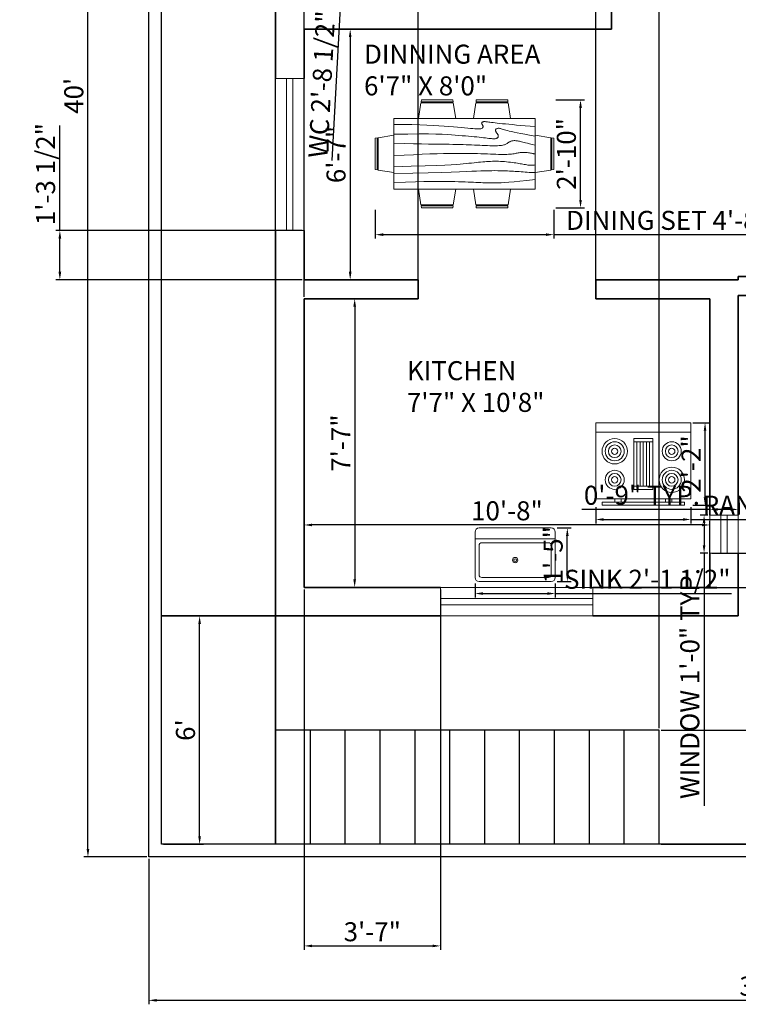
# Model space of a CAD drawing. Units: inches. Extents: x 2117 to 2588, y 1610 to 2201.
# Tile 1 of 4: x 2117 to 2344, y 1610 to 1920. Entities that reach past the tile are written whole.
import ezdxf

# ---------------------------------------------------------------- set-up
doc = ezdxf.new("R2010")
doc.units = ezdxf.units.IN
for name, color, linetype, lineweight in [('A-ANNO-DIMS', 2, 'Continuous', 18), ('A-AREA-IDEN', 7, 'Continuous', 25), ('A-EQPM', 8, 'Continuous', 18), ('A-FLOR-FIXT', 9, 'Continuous', 18), ('A-FLOR-STRS', 7, 'Continuous', 25), ('A-FURN', 8, 'Continuous', 18), ('A-WALL', 7, 'Continuous', 35), ('C-PROP', 7, 'Continuous', 30), ('WINDOW', 150, 'Continuous', 18)]:
    doc.layers.add(name, color=color, linetype=linetype, lineweight=lineweight)
doc.styles.get("Standard").update_dxf_attribs({"font": 'arial.ttf'})
doc.dimstyles.new('ISO-25', dxfattribs={"dimtxt": 6, "dimasz": 2.5, "dimexe": 1.25, "dimexo": 0.625, "dimtad": 1, "dimlunit": 3, "dimtxsty": 'Standard', "dimcen": 2.5, "dimadec": 0, "dimazin": 0, "dimtfac": 1, "dimtmove": 0, "dimatfit": 3, "dimfxl": 1, "dimarcsym": 0})

# ---------------------------------------------------------------- blocks, each defined once
blk = doc.blocks.new('*D5')
at = {"layer": 'A-ANNO-DIMS', "color": 0, "lineweight": -2, "transparency": 16777216}
for p, q in [((2207.7, 1917.03), (2222.87, 1917.03)), ((2221.62, 1914.53), (2221.62, 1840.53)), ((2207.7, 1838.03), (2222.87, 1838.03))]:
    blk.add_line(p, q, dxfattribs=at)
at = {"layer": 'A-ANNO-DIMS', "color": 0, "transparency": 16777216}
for points in [[(2221.21, 1914.53), (2222.04, 1914.53), (2221.62, 1917.03)], [(2221.21, 1840.53), (2222.04, 1840.53), (2221.62, 1838.03)]]:
    blk.add_solid(points, dxfattribs=at)
at = {"layer": 'Defpoints', "color": 0, "transparency": 16777216}
for p in [(2207.08, 1917.03), (2207.08, 1838.03), (2221.62, 1838.03)]:
    blk.add_point(p, dxfattribs=at)
at = {"layer": 'A-ANNO-DIMS', "color": 0, "transparency": 16777216, "insert": (2217.93, 1877.53), "char_height": 6, "attachment_point": 5, "rotation": 90}
blk.add_mtext('6\'-7"', dxfattribs=at)
blk = doc.blocks.new('*D6')
at = {"layer": 'A-ANNO-DIMS', "color": 0, "lineweight": -2, "transparency": 16777216}
for p, q in [((2207.7, 1832.03), (2224.29, 1832.03)), ((2223.04, 1829.53), (2223.04, 1743.53)), ((2207.7, 1741.03), (2224.29, 1741.03))]:
    blk.add_line(p, q, dxfattribs=at)
at = {"layer": 'A-ANNO-DIMS', "color": 0, "transparency": 16777216}
for points in [[(2222.62, 1829.53), (2223.45, 1829.53), (2223.04, 1832.03)], [(2222.62, 1743.53), (2223.45, 1743.53), (2223.04, 1741.03)]]:
    blk.add_solid(points, dxfattribs=at)
at = {"layer": 'Defpoints', "color": 0, "transparency": 16777216}
for p in [(2207.08, 1832.03), (2207.08, 1741.03), (2223.04, 1741.03)]:
    blk.add_point(p, dxfattribs=at)
at = {"layer": 'A-ANNO-DIMS', "color": 0, "transparency": 16777216, "insert": (2219.41, 1786.53), "char_height": 6, "attachment_point": 5, "rotation": 90}
blk.add_mtext('7\'-7"', dxfattribs=at)
blk = doc.blocks.new('*D8')
at = {"layer": 'A-ANNO-DIMS', "color": 0, "lineweight": -2, "transparency": 16777216}
for p, q in [((2162.7, 1732.03), (2175.37, 1732.03)), ((2174.12, 1662.53), (2174.12, 1729.53)), ((2162.7, 1660.03), (2175.37, 1660.03))]:
    blk.add_line(p, q, dxfattribs=at)
at = {"layer": 'A-ANNO-DIMS', "color": 0, "transparency": 16777216}
for points in [[(2173.7, 1729.53), (2174.53, 1729.53), (2174.12, 1732.03)], [(2173.7, 1662.53), (2174.53, 1662.53), (2174.12, 1660.03)]]:
    blk.add_solid(points, dxfattribs=at)
at = {"layer": 'Defpoints', "color": 0, "transparency": 16777216}
for p in [(2162.08, 1732.03), (2174.12, 1732.03), (2162.08, 1660.03)]:
    blk.add_point(p, dxfattribs=at)
at = {"layer": 'A-ANNO-DIMS', "color": 0, "transparency": 16777216, "insert": (2170.43, 1696.03), "char_height": 6, "attachment_point": 5, "rotation": 90}
blk.add_mtext("6'", dxfattribs=at)
blk = doc.blocks.new('*D15')
at = {"layer": 'A-ANNO-DIMS', "color": 0, "lineweight": -2, "transparency": 16777216}
for p, q in [((2207.08, 1741.65), (2207.08, 1761.96)), ((2332.58, 1760.71), (2209.58, 1760.71)), ((2335.08, 1741.65), (2335.08, 1761.96))]:
    blk.add_line(p, q, dxfattribs=at)
at = {"layer": 'A-ANNO-DIMS', "color": 0, "transparency": 16777216}
for points in [[(2209.58, 1761.13), (2209.58, 1760.29), (2207.08, 1760.71)], [(2332.58, 1761.13), (2332.58, 1760.29), (2335.08, 1760.71)]]:
    blk.add_solid(points, dxfattribs=at)
at = {"layer": 'Defpoints', "color": 0, "transparency": 16777216}
for p in [(2207.08, 1760.71), (2207.08, 1741.03), (2335.08, 1741.03)]:
    blk.add_point(p, dxfattribs=at)
at = {"layer": 'A-ANNO-DIMS', "color": 0, "transparency": 16777216, "insert": (2271.08, 1764.4), "char_height": 6, "attachment_point": 5}
blk.add_mtext('10\'-8"', dxfattribs=at)
blk = doc.blocks.new('Dining Set - 36 x 72 in.')
for p, q in [((-22.2343, 26.00059), (-23.4847, 17.99762)), ((-22.2304, 26), (-5.7608, 26)), ((-22, 27.5), (-22.1562, 26.50042)), ((-5.8416, 26.5), (-22.1534, 26.5)), ((-22, 27.5), (-6, 27.5)), ((-5.8437, 26.49966), (-6, 27.5)), ((-4.5152, 17.99762), (-5.7655, 25.99926)), ((5.7657, 26.00059), (4.5153, 17.99762)), ((5.7696, 26), (22.2392, 26)), ((6, 27.5), (5.8438, 26.50042)), ((22.1584, 26.5), (5.8466, 26.5)), ((6, 27.5), (22, 27.5)), ((22.1563, 26.49966), (22, 27.5)), ((23.4848, 17.99762), (22.2345, 25.99926)), ((36, 18), (-36, 18)), ((-36, 18), (-36, -18)), ((36, -18), (36, 18)), ((-45.5, 8), (-44.5004, 8.15617)), ((-45.5, 8), (-45.5, -8)), ((-44.5, -8.15843), (-44.5, 8.15338)), ((-44.0006, 8.23428), (-35.9976, 9.48474)), ((-44, 8.23041), (-44, -8.23915)), ((44.0006, 8.23428), (35.9976, 9.48474)), ((44, 8.23041), (44, -8.23915)), ((44.5, -8.15843), (44.5, 8.15338)), ((45.5, 8), (44.5005, 8.15617)), ((45.5, 8), (45.5, -8)), ((-44.4997, -8.15631), (-45.5, -8)), ((-35.9976, -9.48476), (-43.9993, -8.2345)), ((35.9976, -9.48476), (43.9993, -8.2345)), ((44.4997, -8.15631), (45.5, -8)), ((-36, -18), (36, -18)), ((-22.2343, -26.0006), (-23.4847, -17.99762)), ((-4.5152, -17.99762), (-5.7655, -25.99928)), ((5.7657, -26.0006), (4.5153, -17.99762)), ((23.4848, -17.99762), (22.2345, -25.99928)), ((-22.2304, -26), (-5.7608, -26)), ((-22, -27.5), (-22.1562, -26.50044)), ((-5.8416, -26.5), (-22.1534, -26.5)), ((-22, -27.5), (-6, -27.5)), ((-5.8437, -26.49967), (-6, -27.5)), ((5.7696, -26), (22.2392, -26)), ((6, -27.5), (5.8438, -26.50044)), ((22.1584, -26.5), (5.8466, -26.5)), ((6, -27.5), (22, -27.5)), ((22.1563, -26.49967), (22, -27.5))]:
    blk.add_line(p, q)
for points in [[(-36, 15), (-31.1772, 14.97754), (-26.8079, 14.91406), (-22.8538, 14.81543), (-19.276, 14.6875), (-16.0362, 14.53613), (-13.0957, 14.36718), (-10.4159, 14.18652), (-7.9583, 14), (-5.6904, 13.81315), (-3.6035, 13.63021), (-1.6954, 13.45508), (0.0365, 13.29166), (1.5945, 13.14388), (2.9811, 13.01562), (4.1988, 12.9108), (5.25, 12.83333), (6.1393, 12.78613), (6.8802, 12.76823), (7.4883, 12.77767), (7.9792, 12.8125), (8.3685, 12.87077), (8.6719, 12.95052), (8.9049, 13.0498), (9.0833, 13.16666), (9.2205, 13.29899), (9.3216, 13.44401), (9.3895, 13.59879), (9.4271, 13.76041), (9.4373, 13.92594), (9.4232, 14.09245), (9.3875, 14.257), (9.3333, 14.41666), (9.2638, 14.56917), (9.1836, 14.71484), (9.0975, 14.85465), (9.0104, 14.98958), (8.9272, 15.1206), (8.8529, 15.2487), (8.7922, 15.37483), (8.75, 15.5), (8.7305, 15.62467), (8.7344, 15.74739), (8.7617, 15.86621), (8.8125, 15.97916), (8.8867, 16.08431), (8.9844, 16.17968), (9.1055, 16.26334), (9.25, 16.33333), (9.4189, 16.38802), (9.6172, 16.42708), (9.8506, 16.45052), (10.125, 16.45833), (10.4463, 16.45052), (10.8203, 16.42708), (11.2529, 16.38802), (11.75, 16.33333), (12.3184, 16.26318), (12.9694, 16.17838), (13.7151, 16.07991), (14.5677, 15.96875), (15.5395, 15.84586), (16.6426, 15.71224), (17.8893, 15.56884), (19.2917, 15.41666), (20.859, 15.25667), (22.5879, 15.08984), (24.4721, 14.91715), (26.5052, 14.73958), (28.6809, 14.5581), (30.9929, 14.3737), (33.4347, 14.18733), (36, 14)], [(-36, 10), (-28.9766, 10.14274), (-23.1725, 10.20442), (-18.4241, 10.19775), (-14.5677, 10.13541), (-11.4399, 10.03011), (-8.877, 9.89453), (-6.7154, 9.74137), (-4.7917, 9.58333), (-2.9698, 9.43082), (-1.2246, 9.28515), (0.4415, 9.14534), (2.026, 9.01041), (3.5266, 8.87939), (4.9408, 8.7513), (6.266, 8.62516), (7.5, 8.5), (8.6411, 8.37549), (9.6914, 8.2539), (10.6538, 8.13818), (11.5312, 8.03125), (12.3267, 7.93603), (13.043, 7.85547), (13.6831, 7.79248), (14.25, 7.75), (14.7471, 7.7303), (15.1797, 7.73307), (15.5537, 7.75732), (15.875, 7.80208), (16.1494, 7.86637), (16.3828, 7.94922), (16.5811, 8.04964), (16.75, 8.16666), (16.8944, 8.29915), (17.0143, 8.44531), (17.1089, 8.60319), (17.1771, 8.77083), (17.218, 8.94629), (17.2305, 9.1276), (17.2137, 9.31282), (17.1667, 9.5), (17.0895, 9.6875), (16.987, 9.875), (16.8649, 10.0625), (16.7292, 10.25), (16.5856, 10.4375), (16.4401, 10.625), (16.2985, 10.8125), (16.1667, 11), (16.05, 11.18733), (15.9518, 11.3737), (15.8752, 11.5581), (15.8229, 11.73958), (15.798, 11.91715), (15.8034, 12.08984), (15.842, 12.25667), (15.9167, 12.41666), (16.0295, 12.56836), (16.1784, 12.70833), (16.3605, 12.83268), (16.5729, 12.9375), (16.8127, 13.01888), (17.0768, 13.07291), (17.3625, 13.0957), (17.6667, 13.08333), (17.9894, 13.03312), (18.3418, 12.94726), (18.7382, 12.82918), (19.1927, 12.68229), (19.7195, 12.51001), (20.3327, 12.31575), (21.0465, 12.10294), (21.875, 11.875), (22.8357, 11.63354), (23.959, 11.37304), (25.2786, 11.08618), (26.8282, 10.76562), (28.6414, 10.40405), (30.752, 9.99414), (33.1936, 9.52856), (36, 9)], [(-36, 5.5), (-30.7157, 5.3348), (-26.069, 5.20963), (-21.9946, 5.11767), (-18.4271, 5.05208), (-15.3009, 5.00602), (-12.5508, 4.97265), (-10.1112, 4.94515), (-7.9167, 4.91666), (-5.909, 4.88167), (-4.0586, 4.83984), (-2.3429, 4.79215), (-0.7396, 4.73958), (0.7739, 4.6831), (2.22, 4.6237), (3.6213, 4.56233), (5, 4.5), (6.373, 4.43782), (7.7344, 4.3776), (9.0723, 4.32129), (10.375, 4.27083), (11.6309, 4.22819), (12.8281, 4.19531), (13.9551, 4.17415), (15, 4.16666), (15.954, 4.17448), (16.819, 4.19791), (17.6001, 4.23698), (18.3021, 4.29166), (18.9299, 4.36198), (19.4883, 4.44791), (19.9823, 4.54948), (20.4167, 4.66666), (20.7969, 4.79899), (21.1302, 4.94401), (21.4245, 5.09879), (21.6875, 5.26041), (21.9271, 5.42594), (22.1511, 5.59245), (22.3672, 5.757), (22.5834, 5.91666), (22.8065, 6.06868), (23.0404, 6.21093), (23.2879, 6.34147), (23.5521, 6.45833), (23.8358, 6.55957), (24.142, 6.64323), (24.4735, 6.70735), (24.8334, 6.75), (25.2235, 6.76969), (25.642, 6.76692), (26.0858, 6.74267), (26.5521, 6.69791), (27.0379, 6.63362), (27.5404, 6.55078), (28.0565, 6.45036), (28.5834, 6.33333), (29.1242, 6.19987), (29.7071, 6.04687), (30.3661, 5.87044), (31.1354, 5.66666), (32.0493, 5.43164), (33.142, 5.16146), (34.4475, 4.85221), (36, 4.5)], [(-36, -1), (-30.7915, -0.6591), (-26.0195, -0.38216), (-21.6519, -0.16284), (-17.6563, 0.00521), (-14.0005, 0.12833), (-10.6523, 0.21289), (-7.5796, 0.26522), (-4.75, 0.29166), (-2.134, 0.29793), (0.2878, 0.28711), (2.5317, 0.26163), (4.6146, 0.22396), (6.5529, 0.17651), (8.3633, 0.12174), (10.0623, 0.06209), (11.6667, 0), (13.1899, -0.06201), (14.6341, -0.1211), (15.9982, -0.17432), (17.2813, -0.21875), (18.4823, -0.25147), (19.6003, -0.26953), (20.6343, -0.27002), (21.5834, -0.25), (22.4481, -0.20768), (23.2357, -0.14584), (23.9549, -0.06836), (24.6146, 0.02083), (25.2235, 0.11784), (25.7904, 0.21875), (26.3241, 0.31966), (26.8334, 0.41666), (27.3265, 0.50618), (27.8099, 0.58593), (28.2894, 0.65397), (28.7709, 0.70833), (29.2601, 0.74707), (29.763, 0.76823), (30.2855, 0.76985), (30.8334, 0.75), (31.4088, 0.70784), (31.9994, 0.64713), (32.589, 0.57275), (33.1615, 0.48958), (33.7008, 0.4025), (34.1908, 0.3164), (34.6153, 0.23616), (34.9584, 0.16666), (35.2099, 0.11165), (35.3848, 0.07031), (35.504, 0.04069), (35.5886, 0.02083), (35.6594, 0.00879), (35.7377, 0.0026), (35.8442, 0.00032), (36, 0)], [(-36, -6.5), (-27.1843, -6.31267), (-20.084, -6.1263), (-14.469, -5.9419), (-10.1094, -5.76042), (-6.7752, -5.58285), (-4.2363, -5.41016), (-2.2629, -5.24333), (-0.625, -5.08334), (0.8708, -4.93099), (2.2715, -4.78646), (3.5872, -4.64974), (4.8281, -4.52084), (6.0046, -4.39974), (7.127, -4.28646), (8.2053, -4.18099), (9.25, -4.08334), (10.2705, -3.99382), (11.2734, -3.91407), (12.2647, -3.84603), (13.25, -3.79167), (14.2354, -3.75293), (15.2266, -3.73177), (16.2295, -3.73015), (17.25, -3.75), (18.2912, -3.79248), (19.3451, -3.85547), (20.4009, -3.93604), (21.4479, -4.03125), (22.4754, -4.13819), (23.4727, -4.25391), (24.4289, -4.37549), (25.3334, -4.5), (26.1785, -4.62492), (26.9694, -4.74935), (27.7145, -4.87281), (28.4219, -4.99479), (29.1, -5.11483), (29.7572, -5.23242), (30.4016, -5.34709), (31.0417, -5.45834), (31.6837, -5.56437), (32.3262, -5.65821), (32.9658, -5.73153), (33.599, -5.77604), (34.2224, -5.78345), (34.8327, -5.74545), (35.4264, -5.65373), (36, -5.5)], [(-36, -10), (-26.4022, -9.81299), (-18.4675, -9.62891), (-11.9839, -9.45069), (-6.7396, -9.28125), (-2.5226, -9.12354), (0.8789, -8.98047), (3.6769, -8.85498), (6.0833, -8.75), (8.2767, -8.66765), (10.3021, -8.60677), (12.1712, -8.56543), (13.8958, -8.54167), (15.4876, -8.53353), (16.9583, -8.53907), (18.3197, -8.55632), (19.5834, -8.58334), (20.7616, -8.61841), (21.8685, -8.66081), (22.9188, -8.71004), (23.9271, -8.76563), (24.9081, -8.82707), (25.8763, -8.89388), (26.8465, -8.96558), (27.8334, -9.04167), (28.8474, -9.12118), (29.8828, -9.20117), (30.93, -9.27824), (31.9792, -9.34896), (33.0205, -9.40991), (34.0443, -9.45768), (35.0407, -9.48885), (36, -9.5)], [(-36, -14.5), (-30.0881, -14.33513), (-25.0332, -14.21224), (-20.7312, -14.12647), (-17.0781, -14.07292), (-13.97, -14.04671), (-11.3027, -14.04297), (-8.9724, -14.05681), (-6.875, -14.08334), (-4.9224, -14.11833), (-3.0905, -14.16016), (-1.3709, -14.20785), (0.2448, -14.26042), (1.7647, -14.3169), (3.1973, -14.3763), (4.5507, -14.43767), (5.8333, -14.5), (7.0554, -14.5621), (8.235, -14.62175), (9.3922, -14.67652), (10.5469, -14.72396), (11.7192, -14.76164), (12.929, -14.78711), (14.1965, -14.79794), (15.5417, -14.79167), (16.9933, -14.76424), (18.6152, -14.70508), (20.4804, -14.60197), (22.6615, -14.44271), (25.2312, -14.21509), (28.2624, -13.9069), (31.8277, -13.50594), (36, -13)]]:
    blk.add_lwpolyline(points)
blk = doc.blocks.new('Range-Oven - 30 in top')
for p, q in [((0, -3), (30, -3)), ((12, -6), (18, -6)), ((13, -20), (13, -6)), ((14, -6), (14, -20)), ((15, -20), (15, -6)), ((16, -6), (16, -20)), ((17, -20), (17, -6)), ((18, -20), (12, -20)), ((6, -24), (6, -25)), ((8, -25), (8, -24)), ((22, -25), (22, -24)), ((24, -24), (24, -25))]:
    blk.add_line(p, q)
for points in [[(0, -24), (0, 0), (30, 0), (30, -24)], [(12, -21), (12, -5), (18, -5), (18, -21)], [(2, -26), (2, -25), (28, -25), (28, -26)]]:
    blk.add_lwpolyline(points, close=True)
for centre, radius in [((6, -9), 4), ((6, -9), 3), ((24, -9), 3), ((6, -9), 2), ((6, -9), 1), ((24, -9), 2), ((24, -9), 1), ((6, -18), 3), ((24, -18), 4), ((24, -18), 3), ((6, -18), 2), ((6, -18), 1), ((24, -18), 2), ((24, -18), 1)]:
    blk.add_circle(centre, radius)
blk = doc.blocks.new('Sink-single - 30 in top')
blk.add_line((-15, -3.999996), (15, -3.999996))
for points in [[(-13.5, 0), (13.5, 0)], [(-15, -18.499996), (-15, -1.5)], [(15, -1.5), (15, -18.499996)], [(-13.5, -17.499996), (-13.5, -6.499996)], [(-12.5, -5.499996), (12.5, -5.499996)], [(13.5, -6.499996), (13.5, -17.499996)], [(13.5, -19.999996), (-13.5, -19.999996)], [(12.5, -18.499996), (-12.5, -18.499996)]]:
    blk.add_lwpolyline(points)
for radius in [1, 0.5]:
    blk.add_circle((0, -11.999996), radius)
for centre, radius, start, end in [((-13.5, -1.5), 1.5, 90, 180), ((13.5, -1.5), 1.5, 0, 90), ((-12.5, -6.499996), 1, 90, 180), ((12.5, -6.499996), 1, 0, 90), ((-12.5, -17.499996), 1, 180, 270), ((12.5, -17.499996), 1, 270, 0), ((-13.5, -18.499996), 1.5, 180, 270), ((13.5, -18.499996), 1.5, 270, 0)]:
    blk.add_arc(centre, radius, start, end)
blk = doc.blocks.new('*D32')
at = {"layer": 'A-ANNO-DIMS', "color": 0, "lineweight": -2, "transparency": 16777216}
for p, q in [((2158.08, 1655.4), (2158.08, 1609.57)), ((2542.08, 1655.4), (2542.08, 1609.57)), ((2539.58, 1610.82), (2160.58, 1610.82))]:
    blk.add_line(p, q, dxfattribs=at)
at = {"layer": 'A-ANNO-DIMS', "color": 0, "transparency": 16777216}
for points in [[(2160.58, 1611.24), (2160.58, 1610.4), (2158.08, 1610.82)], [(2539.58, 1611.24), (2539.58, 1610.4), (2542.08, 1610.82)]]:
    blk.add_solid(points, dxfattribs=at)
at = {"layer": 'Defpoints', "color": 0, "transparency": 16777216}
for p in [(2158.08, 1656.03), (2542.08, 1656.03), (2158.08, 1610.82)]:
    blk.add_point(p, dxfattribs=at)
at = {"layer": 'A-ANNO-DIMS', "color": 0, "transparency": 16777216, "insert": (2350.08, 1614.51), "char_height": 6, "attachment_point": 5}
blk.add_mtext("32'", dxfattribs=at)
blk = doc.blocks.new('*D33')
at = {"layer": 'A-ANNO-DIMS', "color": 0, "lineweight": -2, "transparency": 16777216}
for p, q in [((2157.45, 2136.03), (2137.63, 2136.03)), ((2138.88, 1658.53), (2138.88, 2133.53)), ((2157.45, 1656.03), (2137.63, 1656.03))]:
    blk.add_line(p, q, dxfattribs=at)
at = {"layer": 'A-ANNO-DIMS', "color": 0, "transparency": 16777216}
for points in [[(2138.47, 2133.53), (2139.3, 2133.53), (2138.88, 2136.03)], [(2138.47, 1658.53), (2139.3, 1658.53), (2138.88, 1656.03)]]:
    blk.add_solid(points, dxfattribs=at)
at = {"layer": 'Defpoints', "color": 0, "transparency": 16777216}
for p in [(2138.88, 2136.03), (2158.08, 2136.03), (2158.08, 1656.03)]:
    blk.add_point(p, dxfattribs=at)
at = {"layer": 'A-ANNO-DIMS', "color": 0, "transparency": 16777216, "insert": (2135.2, 1896.03), "char_height": 6, "attachment_point": 5, "rotation": 90}
blk.add_mtext("40'", dxfattribs=at)
blk = doc.blocks.new('WIN-48IN-9IN-WALL')
for p, q in [((9, 48), (0, 48)), ((0, 0), (0, 48)), ((3.5, 0), (3.5, 48)), ((5.5, 0), (5.5, 48)), ((9, 0), (9, 48)), ((9, 0), (0, 0))]:
    blk.add_line(p, q)
blk = doc.blocks.new('WIN-12IN-9IN-WALL')
for p, q in [((9, 12), (0, 12)), ((0, 0), (0, 12)), ((3.5, 0), (3.5, 12)), ((5.5, 0), (5.5, 12)), ((9, 0), (9, 12)), ((9, 0), (0, 0))]:
    blk.add_line(p, q)
blk = doc.blocks.new('*D39')
at = {"layer": 'A-ANNO-DIMS', "color": 0, "lineweight": -2, "transparency": 16777216}
for p, q in [((2334.45, 1763.81), (2332.03, 1763.81)), ((2333.28, 1761.31), (2333.28, 1754.31)), ((2334.45, 1751.81), (2332.03, 1751.81)), ((2333.28, 1751.81), (2333.28, 1672.13))]:
    blk.add_line(p, q, dxfattribs=at)
at = {"layer": 'A-ANNO-DIMS', "color": 0, "transparency": 16777216}
for points in [[(2332.86, 1761.31), (2333.69, 1761.31), (2333.28, 1763.81)], [(2332.86, 1754.31), (2333.69, 1754.31), (2333.28, 1751.81)]]:
    blk.add_solid(points, dxfattribs=at)
at = {"layer": 'Defpoints', "color": 0, "transparency": 16777216}
for p in [(2335.08, 1763.81), (2333.28, 1751.81), (2335.08, 1751.81)]:
    blk.add_point(p, dxfattribs=at)
at = {"layer": 'A-ANNO-DIMS', "color": 0, "transparency": 16777216, "insert": (2329.55, 1710.72), "char_height": 6, "attachment_point": 5, "rotation": 90}
blk.add_mtext('WINDOW 1\'-0" TYP.', dxfattribs=at)
blk = doc.blocks.new('*D40')
at = {"layer": 'A-ANNO-DIMS', "color": 0, "lineweight": -2, "transparency": 16777216}
for p, q in [((2335.08, 1764.43), (2335.08, 1766.86)), ((2344.08, 1764.43), (2344.08, 1766.86)), ((2335.08, 1765.61), (2294.75, 1765.61)), ((2341.58, 1765.61), (2337.58, 1765.61))]:
    blk.add_line(p, q, dxfattribs=at)
at = {"layer": 'A-ANNO-DIMS', "color": 0, "transparency": 16777216}
for points in [[(2337.58, 1766.02), (2337.58, 1765.19), (2335.08, 1765.61)], [(2341.58, 1766.02), (2341.58, 1765.19), (2344.08, 1765.61)]]:
    blk.add_solid(points, dxfattribs=at)
at = {"layer": 'Defpoints', "color": 0, "transparency": 16777216}
for p in [(2335.08, 1765.61), (2335.08, 1763.81), (2344.08, 1763.81)]:
    blk.add_point(p, dxfattribs=at)
at = {"layer": 'A-ANNO-DIMS', "color": 0, "transparency": 16777216, "insert": (2313.66, 1769.3), "char_height": 6, "attachment_point": 5}
blk.add_mtext('0\'-9" TYP.', dxfattribs=at)
blk = doc.blocks.new('*D45')
at = {"layer": 'A-ANNO-DIMS', "color": 0, "lineweight": -2, "transparency": 16777216}
for p, q in [((2224.57, 1957.8), (2219.1, 1958.1)), ((2220.21, 1955.54), (2218.73, 1928.23)), ((2218.6, 1925.73), (2215.87, 1875.58)), ((2222.82, 1925.5), (2217.35, 1925.8))]:
    blk.add_line(p, q, dxfattribs=at)
at = {"layer": 'A-ANNO-DIMS', "color": 0, "transparency": 16777216}
for points in [[(2219.8, 1955.56), (2220.63, 1955.51), (2220.35, 1958.03)], [(2218.32, 1928.25), (2219.15, 1928.2), (2218.6, 1925.73)]]:
    blk.add_solid(points, dxfattribs=at)
at = {"layer": 'Defpoints', "color": 0, "transparency": 16777216}
for p in [(2225.19, 1957.77), (2218.6, 1925.73), (2223.44, 1925.47)]:
    blk.add_point(p, dxfattribs=at)
at = {"layer": 'A-ANNO-DIMS', "color": 0, "transparency": 16777216, "insert": (2213.45, 1899.61), "char_height": 6, "attachment_point": 5, "rotation": 86.894}
blk.add_mtext('WC 2\'-8 1/2"', dxfattribs=at)
blk = doc.blocks.new('*D51')
at = {"layer": 'A-ANNO-DIMS', "color": 0, "lineweight": -2, "transparency": 16777216}
for p, q in [((2229.55, 1860.07), (2229.55, 1851)), ((2285.85, 1860.07), (2285.85, 1851)), ((2232.05, 1852.25), (2283.35, 1852.25)), ((2285.85, 1852.25), (2369.53, 1852.25))]:
    blk.add_line(p, q, dxfattribs=at)
at = {"layer": 'A-ANNO-DIMS', "color": 0, "transparency": 16777216}
for points in [[(2232.05, 1852.67), (2232.05, 1851.83), (2229.55, 1852.25)], [(2283.35, 1852.67), (2283.35, 1851.83), (2285.85, 1852.25)]]:
    blk.add_solid(points, dxfattribs=at)
at = {"layer": 'Defpoints', "color": 0, "transparency": 16777216}
for p in [(2229.55, 1860.69), (2285.85, 1860.69), (2285.85, 1852.25)]:
    blk.add_point(p, dxfattribs=at)
at = {"layer": 'A-ANNO-DIMS', "color": 0, "transparency": 16777216, "insert": (2328.94, 1855.98), "char_height": 6, "attachment_point": 5}
blk.add_mtext('DINING SET 4\'-8 1/2"', dxfattribs=at)
blk = doc.blocks.new('*D52')
at = {"layer": 'A-ANNO-DIMS', "color": 0, "lineweight": -2, "transparency": 16777216}
for p, q in [((2286.47, 1894.72), (2295.54, 1894.72)), ((2294.29, 1863.19), (2294.29, 1892.22)), ((2286.47, 1860.69), (2295.54, 1860.69))]:
    blk.add_line(p, q, dxfattribs=at)
at = {"layer": 'A-ANNO-DIMS', "color": 0, "transparency": 16777216}
for points in [[(2293.88, 1892.22), (2294.71, 1892.22), (2294.29, 1894.72)], [(2293.88, 1863.19), (2294.71, 1863.19), (2294.29, 1860.69)]]:
    blk.add_solid(points, dxfattribs=at)
at = {"layer": 'Defpoints', "color": 0, "transparency": 16777216}
for p in [(2285.85, 1894.72), (2294.29, 1894.72), (2285.85, 1860.69)]:
    blk.add_point(p, dxfattribs=at)
at = {"layer": 'A-ANNO-DIMS', "color": 0, "transparency": 16777216, "insert": (2290.6, 1877.71), "char_height": 6, "attachment_point": 5, "rotation": 90}
blk.add_mtext('2\'-10"', dxfattribs=at)
blk = doc.blocks.new('*D53')
at = {"layer": 'A-ANNO-DIMS', "color": 0, "lineweight": -2, "transparency": 16777216}
for p, q in [((2299.08, 1766.32), (2299.08, 1761.19)), ((2329.08, 1766.32), (2329.08, 1761.19)), ((2301.58, 1762.44), (2326.58, 1762.44)), ((2329.08, 1762.44), (2380.6, 1762.44))]:
    blk.add_line(p, q, dxfattribs=at)
at = {"layer": 'A-ANNO-DIMS', "color": 0, "transparency": 16777216}
for points in [[(2301.58, 1762.86), (2301.58, 1762.02), (2299.08, 1762.44)], [(2326.58, 1762.86), (2326.58, 1762.02), (2329.08, 1762.44)]]:
    blk.add_solid(points, dxfattribs=at)
at = {"layer": 'Defpoints', "color": 0, "transparency": 16777216}
for p in [(2299.08, 1766.94), (2329.08, 1766.94), (2329.08, 1762.44)]:
    blk.add_point(p, dxfattribs=at)
at = {"layer": 'A-ANNO-DIMS', "color": 0, "transparency": 16777216, "insert": (2356.09, 1766.17), "char_height": 6, "attachment_point": 5}
blk.add_mtext('RANGE 2\'-6"', dxfattribs=at)
blk = doc.blocks.new('*D54')
at = {"layer": 'A-ANNO-DIMS', "color": 0, "lineweight": -2, "transparency": 16777216}
for p, q in [((2329.7, 1792.94), (2334.83, 1792.94)), ((2333.58, 1769.44), (2333.58, 1790.44)), ((2329.7, 1766.94), (2334.83, 1766.94))]:
    blk.add_line(p, q, dxfattribs=at)
at = {"layer": 'A-ANNO-DIMS', "color": 0, "transparency": 16777216}
for points in [[(2333.16, 1790.44), (2333.99, 1790.44), (2333.58, 1792.94)], [(2333.16, 1769.44), (2333.99, 1769.44), (2333.58, 1766.94)]]:
    blk.add_solid(points, dxfattribs=at)
at = {"layer": 'Defpoints', "color": 0, "transparency": 16777216}
for p in [(2329.08, 1792.94), (2333.58, 1792.94), (2329.08, 1766.94)]:
    blk.add_point(p, dxfattribs=at)
at = {"layer": 'A-ANNO-DIMS', "color": 0, "transparency": 16777216, "insert": (2329.94, 1779.94), "char_height": 6, "attachment_point": 5, "rotation": 90}
blk.add_mtext('2\'-2"', dxfattribs=at)
blk = doc.blocks.new('*D55')
at = {"layer": 'A-ANNO-DIMS', "color": 0, "lineweight": -2, "transparency": 16777216}
for p, q in [((2261.02, 1742.26), (2261.02, 1737.83)), ((2286.34, 1742.26), (2286.34, 1737.83)), ((2263.52, 1739.08), (2283.84, 1739.08)), ((2286.34, 1739.08), (2341.88, 1739.08))]:
    blk.add_line(p, q, dxfattribs=at)
at = {"layer": 'A-ANNO-DIMS', "color": 0, "transparency": 16777216}
for points in [[(2263.52, 1739.5), (2263.52, 1738.67), (2261.02, 1739.08)], [(2283.84, 1739.5), (2283.84, 1738.67), (2286.34, 1739.08)]]:
    blk.add_solid(points, dxfattribs=at)
at = {"layer": 'Defpoints', "color": 0, "transparency": 16777216}
for p in [(2261.02, 1742.88), (2286.34, 1742.88), (2286.34, 1739.08)]:
    blk.add_point(p, dxfattribs=at)
at = {"layer": 'A-ANNO-DIMS', "color": 0, "transparency": 16777216, "insert": (2315.36, 1742.81), "char_height": 6, "attachment_point": 5}
blk.add_mtext('SINK 2\'-1 1/2"', dxfattribs=at)
blk = doc.blocks.new('*D56')
at = {"layer": 'A-ANNO-DIMS', "color": 0, "lineweight": -2, "transparency": 16777216}
for p, q in [((2286.96, 1759.76), (2291.38, 1759.76)), ((2290.13, 1745.38), (2290.13, 1757.26)), ((2286.96, 1742.88), (2291.38, 1742.88))]:
    blk.add_line(p, q, dxfattribs=at)
at = {"layer": 'A-ANNO-DIMS', "color": 0, "transparency": 16777216}
for points in [[(2289.72, 1757.26), (2290.55, 1757.26), (2290.13, 1759.76)], [(2289.72, 1745.38), (2290.55, 1745.38), (2290.13, 1742.88)]]:
    blk.add_solid(points, dxfattribs=at)
at = {"layer": 'Defpoints', "color": 0, "transparency": 16777216}
for p in [(2286.34, 1759.76), (2290.13, 1759.76), (2286.34, 1742.88)]:
    blk.add_point(p, dxfattribs=at)
at = {"layer": 'A-ANNO-DIMS', "color": 0, "transparency": 16777216, "insert": (2286.44, 1751.32), "char_height": 6, "attachment_point": 5, "rotation": 90}
blk.add_mtext('1\'-5"', dxfattribs=at)
blk = doc.blocks.new('*D58')
at = {"layer": 'A-ANNO-DIMS', "color": 0, "lineweight": -2, "transparency": 16777216}
for p, q in [((2198.08, 1696.65), (2198.08, 2165.33)), ((2200.58, 2164.08), (2316.58, 2164.08)), ((2319.08, 1696.65), (2319.08, 2165.33))]:
    blk.add_line(p, q, dxfattribs=at)
at = {"layer": 'A-ANNO-DIMS', "color": 0, "transparency": 16777216}
for points in [[(2200.58, 2164.5), (2200.58, 2163.66), (2198.08, 2164.08)], [(2316.58, 2164.5), (2316.58, 2163.66), (2319.08, 2164.08)]]:
    blk.add_solid(points, dxfattribs=at)
at = {"layer": 'Defpoints', "color": 0, "transparency": 16777216}
for p in [(2319.08, 2164.08), (2198.08, 1696.03), (2319.08, 1696.03)]:
    blk.add_point(p, dxfattribs=at)
at = {"layer": 'A-ANNO-DIMS', "color": 0, "transparency": 16777216, "insert": (2258.58, 2167.77), "char_height": 6, "attachment_point": 5}
blk.add_mtext('10\'-1"', dxfattribs=at)
blk = doc.blocks.new('*D59')
at = {"layer": 'A-ANNO-DIMS', "color": 0, "lineweight": -2, "transparency": 16777216}
for p, q in [((2319.7, 1696.03), (2571.38, 1696.03)), ((2570.13, 1693.53), (2570.13, 1662.53)), ((2319.7, 1660.03), (2571.38, 1660.03))]:
    blk.add_line(p, q, dxfattribs=at)
at = {"layer": 'A-ANNO-DIMS', "color": 0, "transparency": 16777216}
for points in [[(2569.71, 1693.53), (2570.54, 1693.53), (2570.13, 1696.03)], [(2569.71, 1662.53), (2570.54, 1662.53), (2570.13, 1660.03)]]:
    blk.add_solid(points, dxfattribs=at)
at = {"layer": 'Defpoints', "color": 0, "transparency": 16777216}
for p in [(2319.08, 1696.03), (2319.08, 1660.03), (2570.13, 1660.03)]:
    blk.add_point(p, dxfattribs=at)
at = {"layer": 'A-ANNO-DIMS', "color": 0, "transparency": 16777216, "insert": (2566.44, 1678.03), "char_height": 6, "attachment_point": 5, "rotation": 90}
blk.add_mtext('3\'-0"', dxfattribs=at)
blk = doc.blocks.new('*D60')
at = {"layer": 'A-ANNO-DIMS', "color": 0, "lineweight": -2, "transparency": 16777216}
for p, q in [((2243.08, 1832.65), (2243.08, 2165.33)), ((2245.58, 2164.08), (2296.58, 2164.08)), ((2299.08, 1832.65), (2299.08, 2165.33))]:
    blk.add_line(p, q, dxfattribs=at)
at = {"layer": 'A-ANNO-DIMS', "color": 0, "transparency": 16777216}
for points in [[(2245.58, 2164.5), (2245.58, 2163.66), (2243.08, 2164.08)], [(2296.58, 2164.5), (2296.58, 2163.66), (2299.08, 2164.08)]]:
    blk.add_solid(points, dxfattribs=at)
at = {"layer": 'Defpoints', "color": 0, "transparency": 16777216}
for p in [(2299.08, 2164.08), (2243.08, 1832.03), (2299.08, 1832.03)]:
    blk.add_point(p, dxfattribs=at)
at = {"layer": 'A-ANNO-DIMS', "color": 0, "transparency": 16777216, "insert": (2271.08, 2167.77), "char_height": 6, "attachment_point": 5}
blk.add_mtext('4\'-8"', dxfattribs=at)
blk = doc.blocks.new('*D68')
at = {"layer": 'A-ANNO-DIMS', "color": 0, "lineweight": -2, "transparency": 16777216}
for p, q in [((2207.08, 1740.4), (2207.08, 1626.73)), ((2250.13, 1740.4), (2250.13, 1626.73)), ((2209.58, 1627.98), (2247.63, 1627.98))]:
    blk.add_line(p, q, dxfattribs=at)
at = {"layer": 'A-ANNO-DIMS', "color": 0, "transparency": 16777216}
for points in [[(2209.58, 1628.4), (2209.58, 1627.56), (2207.08, 1627.98)], [(2247.63, 1628.4), (2247.63, 1627.56), (2250.13, 1627.98)]]:
    blk.add_solid(points, dxfattribs=at)
at = {"layer": 'Defpoints', "color": 0, "transparency": 16777216}
for p in [(2207.08, 1741.03), (2250.13, 1741.03), (2250.13, 1627.98)]:
    blk.add_point(p, dxfattribs=at)
at = {"layer": 'A-ANNO-DIMS', "color": 0, "transparency": 16777216, "insert": (2228.6, 1631.67), "char_height": 6, "attachment_point": 5}
blk.add_mtext('3\'-7"', dxfattribs=at)
blk = doc.blocks.new('*D69')
at = {"layer": 'A-ANNO-DIMS', "color": 0, "lineweight": -2, "transparency": 16777216}
for p, q in [((2570.13, 1751.81), (2570.13, 1776.17)), ((2335.7, 1751.81), (2571.38, 1751.81)), ((2570.13, 1743.53), (2570.13, 1749.31)), ((2335.7, 1741.03), (2571.38, 1741.03))]:
    blk.add_line(p, q, dxfattribs=at)
at = {"layer": 'A-ANNO-DIMS', "color": 0, "transparency": 16777216}
for points in [[(2569.71, 1749.31), (2570.54, 1749.31), (2570.13, 1751.81)], [(2569.71, 1743.53), (2570.54, 1743.53), (2570.13, 1741.03)]]:
    blk.add_solid(points, dxfattribs=at)
at = {"layer": 'Defpoints', "color": 0, "transparency": 16777216}
for p in [(2335.08, 1751.81), (2570.13, 1751.81), (2335.08, 1741.03)]:
    blk.add_point(p, dxfattribs=at)
at = {"layer": 'A-ANNO-DIMS', "color": 0, "transparency": 16777216, "insert": (2566.44, 1765.24), "char_height": 6, "attachment_point": 5, "rotation": 90}
blk.add_mtext('0\'-11"', dxfattribs=at)
blk = doc.blocks.new('*D70')
at = {"layer": 'A-ANNO-DIMS', "color": 0, "lineweight": -2, "transparency": 16777216}
for p, q in [((2130.03, 1853.53), (2130.03, 1886.64)), ((2206.45, 1853.53), (2128.78, 1853.53)), ((2130.03, 1840.53), (2130.03, 1851.03)), ((2206.45, 1838.03), (2128.78, 1838.03))]:
    blk.add_line(p, q, dxfattribs=at)
at = {"layer": 'A-ANNO-DIMS', "color": 0, "transparency": 16777216}
for points in [[(2129.61, 1851.03), (2130.44, 1851.03), (2130.03, 1853.53)], [(2129.61, 1840.53), (2130.44, 1840.53), (2130.03, 1838.03)]]:
    blk.add_solid(points, dxfattribs=at)
at = {"layer": 'Defpoints', "color": 0, "transparency": 16777216}
for p in [(2130.03, 1853.53), (2207.08, 1853.53), (2207.08, 1838.03)]:
    blk.add_point(p, dxfattribs=at)
at = {"layer": 'A-ANNO-DIMS', "color": 0, "transparency": 16777216, "insert": (2126.3, 1871.34), "char_height": 6, "attachment_point": 5, "rotation": 90}
blk.add_mtext('1\'-3 1/2"', dxfattribs=at)
blk = doc.blocks.new('*D76')
at = {"layer": 'A-ANNO-DIMS', "color": 0, "lineweight": -2, "transparency": 16777216}
for p, q in [((2207.08, 1832.65), (2207.08, 2165.33)), ((2209.58, 2164.08), (2240.58, 2164.08)), ((2243.08, 1832.65), (2243.08, 2165.33))]:
    blk.add_line(p, q, dxfattribs=at)
at = {"layer": 'A-ANNO-DIMS', "color": 0, "transparency": 16777216}
for points in [[(2209.58, 2164.5), (2209.58, 2163.66), (2207.08, 2164.08)], [(2240.58, 2164.5), (2240.58, 2163.66), (2243.08, 2164.08)]]:
    blk.add_solid(points, dxfattribs=at)
at = {"layer": 'Defpoints', "color": 0, "transparency": 16777216}
for p in [(2243.08, 2164.08), (2207.08, 1832.03), (2243.08, 1832.03)]:
    blk.add_point(p, dxfattribs=at)
at = {"layer": 'A-ANNO-DIMS', "color": 0, "transparency": 16777216, "insert": (2225.08, 2167.77), "char_height": 6, "attachment_point": 5}
blk.add_mtext('3\'-0"', dxfattribs=at)

msp = doc.modelspace()

# ---------------------------------------------------------------- linework, layer by layer
at = {"layer": 'A-FLOR-STRS'}
for p, q in [((2319.076, 1696.029), (2198.076, 1696.029)), ((2209.076, 1660.029), (2209.076, 1696.029)), ((2220.076, 1660.029), (2220.076, 1696.029)), ((2231.076, 1660.029), (2231.076, 1696.029)), ((2242.076, 1660.029), (2242.076, 1696.029)), ((2253.076, 1660.029), (2253.076, 1696.029)), ((2264.076, 1660.029), (2264.076, 1696.029)), ((2275.076, 1660.029), (2275.076, 1696.029)), ((2286.076, 1660.029), (2286.076, 1696.029)), ((2297.076, 1660.029), (2297.076, 1696.029)), ((2308.076, 1660.029), (2308.076, 1696.029)), ((2319.076, 1660.029), (2319.076, 1696.029))]:
    msp.add_line(p, q, dxfattribs=at)
at = {"layer": 'A-WALL'}
for p, q in [((2304.076, 1917.029), (2304.076, 1977.029)), ((2198.076, 1901.529), (2198.076, 1944.029)), ((2207.076, 1917.029), (2304.076, 1917.029)), ((2207.076, 1901.529), (2207.076, 1917.029)), ((2198.076, 1660.029), (2198.076, 1853.529)), ((2207.076, 1838.029), (2207.076, 1853.529)), ((2207.076, 1838.029), (2243.076, 1838.029)), ((2243.076, 1832.029), (2243.076, 1838.029)), ((2299.076, 1832.029), (2299.076, 1838.029)), ((2299.076, 1838.029), (2344.076, 1838.029)), ((2344.076, 1839.029), (2351.076, 1839.029)), ((2344.076, 1838.029), (2344.076, 1839.029)), ((2207.076, 1741.029), (2207.076, 1832.029)), ((2207.076, 1832.029), (2243.076, 1832.029)), ((2299.076, 1832.029), (2335.076, 1832.029)), ((2335.076, 1763.807), (2335.076, 1832.029)), ((2344.076, 1833.029), (2351.076, 1833.029)), ((2351.076, 1833.029), (2344.076, 1833.029)), ((2344.076, 1763.807), (2344.076, 1833.029)), ((2335.076, 1741.029), (2335.076, 1751.807)), ((2344.076, 1732.029), (2344.076, 1751.807)), ((2250.131, 1741.029), (2207.076, 1741.029)), ((2335.076, 1741.029), (2298.131, 1741.029)), ((2250.131, 1732.029), (2162.076, 1732.029)), ((2344.076, 1732.029), (2298.131, 1732.029))]:
    msp.add_line(p, q, dxfattribs=at)
at = {"layer": 'C-PROP'}
for p, q in [((2162.076, 1660.029), (2162.076, 2127.029)), ((2350.076, 1660.029), (2162.076, 1660.029))]:
    msp.add_line(p, q, dxfattribs=at)
msp.add_lwpolyline([(2350.076, 1656.029), (2158.076, 1656.029), (2158.076, 2136.029), (2361.076, 2136.029)], dxfattribs=at)

# ---------------------------------------------------------------- block references
at = {"layer": 'A-EQPM'}
msp.add_blockref('Range-Oven - 30 in top', (2299.076, 1792.941), dxfattribs=at)
at = {"layer": 'A-FLOR-FIXT', "xscale": 0.843779058288721, "yscale": 0.843779058288721, "zscale": 0.843779058288721}
msp.add_blockref('Sink-single - 30 in top', (2273.679, 1759.757), dxfattribs=at)
at = {"layer": 'A-FURN', "xscale": 0.618613975606047, "yscale": 0.618613975606047, "zscale": 0.618613975606047}
msp.add_blockref('Dining Set - 36 x 72 in.', (2257.701, 1877.705), dxfattribs=at)
at = {"layer": 'WINDOW'}
msp.add_blockref('WIN-48IN-9IN-WALL', (2198.076, 1853.529), dxfattribs=at)
for name, p, rotation in [('WIN-12IN-9IN-WALL', (2344.076, 1763.806), 180), ('WIN-48IN-9IN-WALL', (2250.132, 1741.028), 269.9999999999995)]:
    msp.add_blockref(name, p, dxfattribs=dict(at, rotation=rotation))

# ---------------------------------------------------------------- texts
at = {"layer": 'A-AREA-IDEN', "char_height": 6, "attachment_point": 1}
for s, width, insert in [('{\\fArial|b1|i0|c0|p34;DINNING AREA\\P6\'7" X 8\'0"}', 69.80799, (2225.988, 1912.161)), ('{\\fArial|b1|i0|c0|p34;KITCHEN \\P7\'7" X 10\'8"}', 74.29565, (2239.529, 1812.363))]:
    msp.add_mtext_dynamic_manual_height_columns(s, width=width, gutter_width=12.5, heights=[0], dxfattribs=dict(at, insert=insert))

# ---------------------------------------------------------------- dimensions: what is measured, and where the dimension line sits
at = {"layer": 'A-ANNO-DIMS'}
for base, p1, p2, override, picture, middle in [((2319.076, 2164.079), (2198.076, 1696.029), (2319.076, 1696.029), {"dimdec": 1, "dimlfac": 1, "dimrnd": 0, "dimzin": 1, "dimdsep": 46, "dimlunit": 4, "dimfrac": 2}, '*D58', (2258.576, 2167.767)), ((2243.076, 2164.079), (2207.076, 1832.029), (2243.076, 1832.029), {"dimdec": 1, "dimlfac": 1, "dimrnd": 0, "dimzin": 1, "dimdsep": 46, "dimlunit": 4, "dimfrac": 2}, '*D76', (2225.076, 2167.769)), ((2299.076, 2164.079), (2243.076, 1832.029), (2299.076, 1832.029), {"dimdec": 1, "dimlfac": 1, "dimrnd": 0, "dimzin": 1, "dimdsep": 46, "dimlunit": 4, "dimfrac": 2}, '*D60', (2271.076, 2167.767)), ((2207.076, 1760.71), (2335.076, 1741.029), (2207.076, 1741.029), {"dimclrd": 0, "dimclre": 0, "dimclrt": 0}, '*D15', (2271.076, 1764.398)), ((2250.131, 1627.979), (2207.076, 1741.029), (2250.131, 1741.029), {"dimdec": 1, "dimlfac": 1, "dimrnd": 0, "dimzin": 1, "dimdsep": 46, "dimlunit": 4, "dimfrac": 2}, '*D68', (2228.604, 1631.669)), ((2158.076, 1610.819), (2542.076, 1656.029), (2158.076, 1656.029), {"dimclrd": 0, "dimclre": 0, "dimclrt": 0}, '*D32', (2350.076, 1614.509))]:
    dim = msp.add_linear_dim(base=base, p1=p1, p2=p2, dimstyle='ISO-25', override=override, dxfattribs=at)
    dim.commit()
    dim.dimension.update_dxf_attribs({"geometry": picture, "text_midpoint": middle})
for base, p1, p2, override, picture, middle in [((2138.884, 2136.029), (2158.076, 1656.029), (2158.076, 2136.029), {"dimclrd": 0, "dimclre": 0, "dimclrt": 0}, '*D33', (2135.195, 1896.029)), ((2221.622, 1838.029), (2207.076, 1917.029), (2207.076, 1838.029), {"dimclrd": 0, "dimclre": 0, "dimclrt": 0}, '*D5', (2217.934, 1877.529)), ((2294.292, 1894.717), (2285.848, 1860.694), (2285.848, 1894.717), {"dimdec": 1, "dimlfac": 1, "dimrnd": 0, "dimzin": 1, "dimdsep": 46, "dimlunit": 4, "dimfrac": 2}, '*D52', (2290.604, 1877.705)), ((2130.026, 1853.529), (2207.076, 1838.029), (2207.076, 1853.529), {"dimdec": 1, "dimlfac": 1, "dimrnd": 0, "dimzin": 1, "dimdsep": 46, "dimlunit": 4, "dimfrac": 2}, '*D70', (2126.297, 1871.336)), ((2223.035, 1741.029), (2207.076, 1832.029), (2207.076, 1741.029), {"dimclrd": 0, "dimclre": 0, "dimclrt": 0}, '*D6', (2219.41, 1786.529)), ((2333.576, 1792.941), (2329.076, 1766.941), (2329.076, 1792.941), {"dimdec": 1, "dimlfac": 1, "dimrnd": 0, "dimzin": 1, "dimdsep": 46, "dimlunit": 4, "dimfrac": 2}, '*D54', (2329.939, 1779.941)), ((2570.126, 1751.807), (2335.076, 1741.029), (2335.076, 1751.807), {"dimdec": 1, "dimlfac": 1, "dimrnd": 0, "dimzin": 1, "dimdsep": 46, "dimlunit": 4, "dimfrac": 2}, '*D69', (2566.437, 1765.237)), ((2290.133, 1759.757), (2286.336, 1742.882), (2286.336, 1759.757), {"dimdec": 1, "dimlfac": 1, "dimrnd": 0, "dimzin": 1, "dimdsep": 46, "dimlunit": 4, "dimfrac": 2}, '*D56', (2286.445, 1751.32)), ((2174.118, 1732.029), (2162.076, 1660.029), (2162.076, 1732.029), {"dimclrd": 0, "dimclre": 0, "dimclrt": 0}, '*D8', (2170.429, 1696.029)), ((2570.126, 1660.029), (2319.076, 1696.029), (2319.076, 1660.029), {"dimdec": 1, "dimlfac": 1, "dimrnd": 0, "dimzin": 1, "dimdsep": 46, "dimlunit": 4, "dimfrac": 2}, '*D59', (2566.435, 1678.029))]:
    dim = msp.add_linear_dim(base=base, p1=p1, p2=p2, angle=90, dimstyle='ISO-25', override=override, dxfattribs=at)
    dim.commit()
    dim.dimension.update_dxf_attribs({"geometry": picture, "text_midpoint": middle})
for base, p1, p2, angle, text, picture, middle in [((2218.596, 1925.729), (2225.194, 1957.769), (2223.441, 1925.466), 266.89404, 'WC <>', '*D45', (2213.446, 1899.61)), ((2335.076, 1765.607), (2344.076, 1763.807), (2335.076, 1763.807), 180, '<> TYP.', '*D40', (2313.664, 1769.295)), ((2333.276, 1751.807), (2335.076, 1763.807), (2335.076, 1751.807), 270, 'WINDOW <> TYP.', '*D39', (2329.547, 1710.719))]:
    dim = msp.add_linear_dim(base=base, p1=p1, p2=p2, angle=angle, text=text, dimstyle='ISO-25', override={"dimdec": 1, "dimlfac": 1, "dimrnd": 0, "dimzin": 1, "dimdsep": 46, "dimlunit": 4, "dimfrac": 2}, dxfattribs=at)
    dim.commit()
    dim.dimension.update_dxf_attribs({"geometry": picture, "text_midpoint": middle})
for base, p1, p2, text, picture, middle in [((2285.848, 1852.249), (2229.554, 1860.694), (2285.848, 1860.694), 'DINING SET <>', '*D51', (2328.937, 1855.977)), ((2329.076, 1762.441), (2299.076, 1766.941), (2329.076, 1766.941), 'RANGE <>', '*D53', (2356.088, 1766.169)), ((2286.336, 1739.085), (2261.023, 1742.882), (2286.336, 1742.882), 'SINK <>', '*D55', (2315.358, 1742.812))]:
    dim = msp.add_linear_dim(base=base, p1=p1, p2=p2, text=text, dimstyle='ISO-25', override={"dimdec": 1, "dimlfac": 1, "dimrnd": 0, "dimzin": 1, "dimdsep": 46, "dimlunit": 4, "dimfrac": 2}, dxfattribs=at)
    dim.commit()
    dim.dimension.update_dxf_attribs({"geometry": picture, "text_midpoint": middle})

doc.saveas('drawing.dxf')
